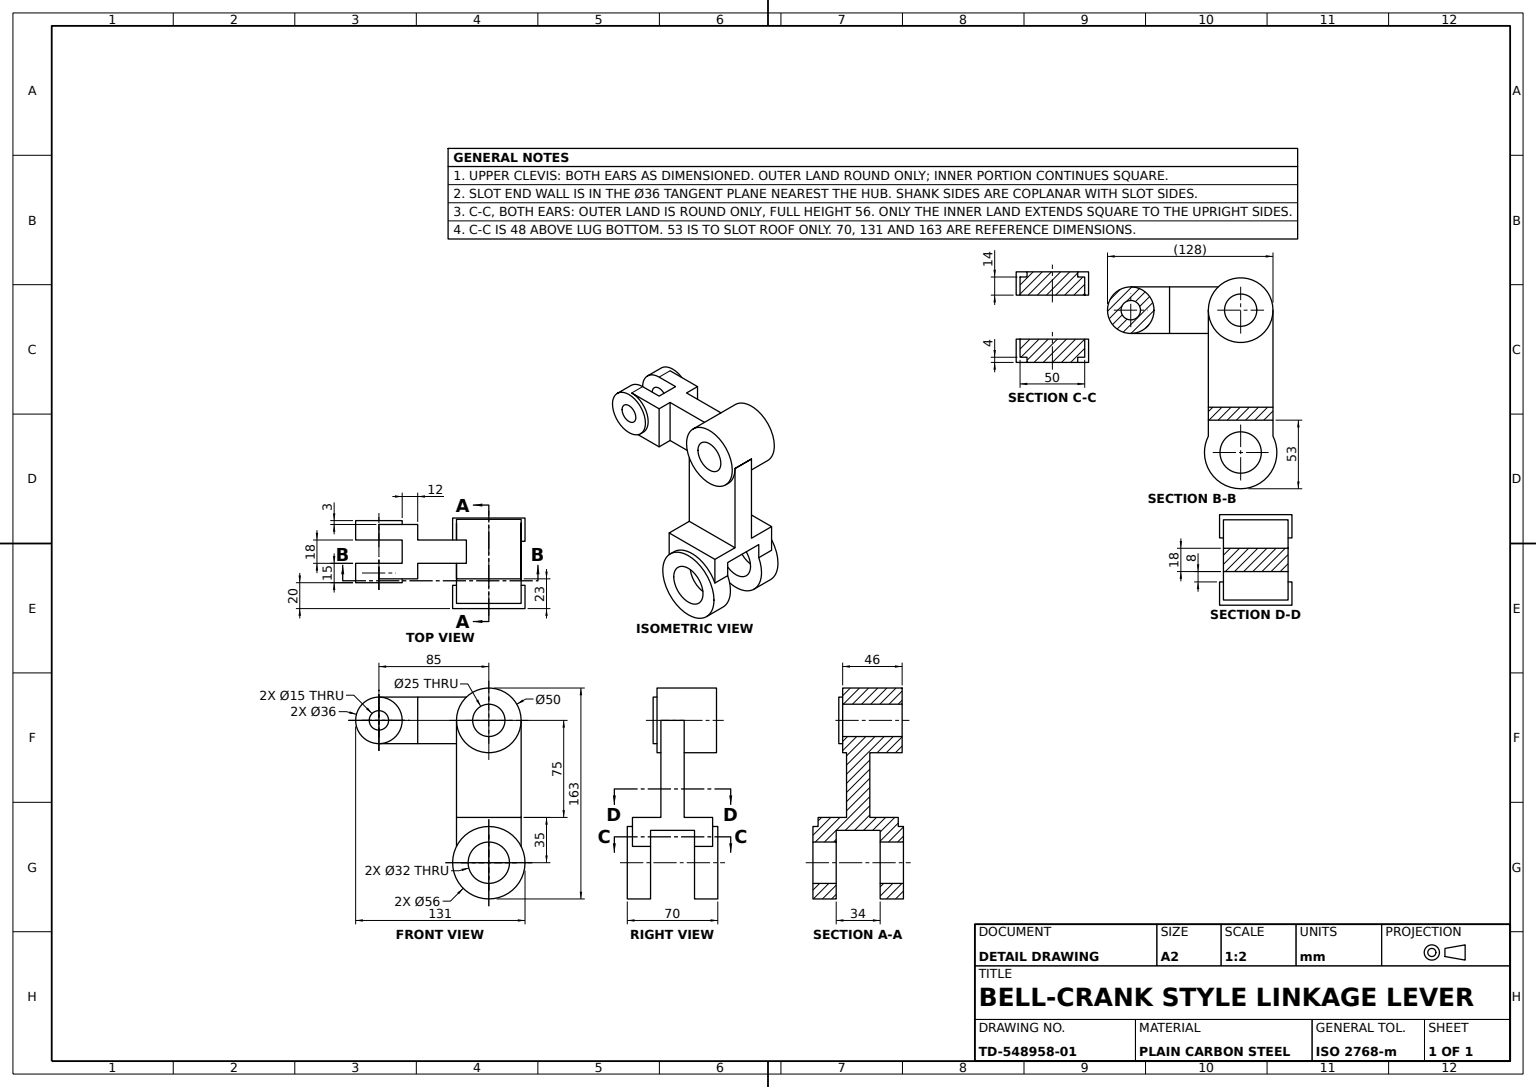
SolidWorks part; units mm, degrees
material "Plain Carbon Steel"
ref_plane "Front Plane" through (0, 0, 0) normal (0, 0, 1) x (1, 0, 0)
ref_plane "Top Plane" through (0, 0, 0) normal (0, 1, 0) x (1, 0, 0)
ref_plane "Right Plane" through (0, 0, 0) normal (1, 0, 0) x (0, 0, -1)
sketch "Front Pivot Eye Sketch" plane through (0, 0, 0) normal (0, 0, 1) x (1, 0, 0)
  circle A0 centre (0, 0) radius 28
  circle A1 centre (0, 0) radius 16
  dimension "D1" = 56
  dimension "D2" = 32
extrude "Front Pivot Eye Ø56xØ32" add sketch "Front Pivot Eye Sketch" against normal blind 18
ref_plane "Plane1" through (0, 0, -52) normal (0, 0, 1) x (1, 0, 0)
sketch "Rear Pivot Eye Sketch" plane through (0, 0, -52) normal (0, 0, 1) x (1, 0, 0)
  circle A0 centre (0, 0) radius 28
  circle A1 centre (0, 0) radius 16
  dimension "D1" = 56
  dimension "D2" = 32
extrude "Rear Pivot Eye Ø56xØ32" add sketch "Rear Pivot Eye Sketch" against normal blind 18 separate body
ref_plane "Plane2" through (0, 35, 0) normal (0, 1, 0) x (1, 0, 0)
sketch "Lower Clevis Block Sketch" plane through (0, 35, 0) normal (0, 1, 0) x (1, 0, 0)
  line L0 (-28, 52) -> (-28, 66)
  line L1 (-28, 70) -> (-28, 52) construction
  line L2 (-28, 66) -> (28, 66)
  line L3 (28, 52) -> (28, 70) construction
  line L4 (28, 66) -> (28, 18)
  line L5 (28, 18) -> (28, 4)
  line L6 (28, 4) -> (-28, 4)
  line L7 (-28, 18) -> (-28, 0) construction
  line L8 (-28, 4) -> (-28, 52)
  dimension "D1" = 48
  dimension "D2" = 48
extrude "Lower Clevis Block 48x48" add sketch "Lower Clevis Block Sketch" against normal blind 18
sketch "Clevis Block Relief Sketch" plane through (0, 0, -4) normal (0, 0, 1) x (1, 0, 0)
  line L0 (-28, 17) -> (-25, 17)
  line L1 (28, 17) -> (25.1243, 17)
  line L2 (-25, 17) -> (-25, 35)
  line L3 (-28, 35) -> (-28, 17)
  line L4 (-28, 17) -> (-28, 35) construction
  line L5 (-28, 17) -> (-22.2486, 17) construction
  line L6 (-28, 35) -> (28, 35) construction
  line L7 (-25, 35) -> (-28, 35)
  line L8 (28, 35) -> (28, 17)
  line L10 (22.2486, 17) -> (28, 17) construction
  line L11 (25.1243, 17) -> (25.0043, 17)
  line L12 (25.0043, 17) -> (25.0043, 35)
  line L13 (25.0043, 35) -> (28, 35)
  dimension "D1" = 3
  dimension "D2" = 2.9957
  dimension "D3" = 2.9957
extrude "Clevis Block Relief Cut" cut sketch "Clevis Block Relief Sketch" against normal through all
sketch "Lower Clevis Slot Sketch" plane through (-25, 0, 0) normal (-1, 0, 0) x (0, 0, 1)
  line L1 (-52, 17) -> (-18, 17)
  line L2 (-52, 17) -> (-52, 25)
  line L3 (-52, 25) -> (-18, 25)
  line L4 (-18, 17) -> (-18, 25)
  dimension "D1" = 34
  dimension "D2" = 8
extrude "Lower Clevis Slot 34x8" cut sketch "Lower Clevis Slot Sketch" against normal through all
sketch "Lower Web Plate Sketch" plane through (0, 17, 0) normal (0, -1, 0) x (1, 0, 0)
  line L0 (22.2486, -4) -> (22.2486, -18) construction
  line L1 (-25, -66) -> (-22.2486, -66)
  line L2 (-25, -66) -> (-25, -52)
  line L3 (-25, -52) -> (-22.2486, -52)
  line L4 (-22.2486, -66) -> (-22.2486, -52)
  line L5 (-25, -18) -> (-22.2486, -18)
  line L6 (-25, -18) -> (-25, -4)
  line L7 (-25, -4) -> (-22.2486, -4)
  line L8 (-22.2486, -18) -> (-22.2486, -4)
  line L9 (22.2486, -4) -> (25.0043, -4)
  line L10 (22.2486, -4) -> (22.2486, -18)
  line L11 (22.2486, -18) -> (25.0043, -18)
  line L12 (25.0043, -4) -> (25.0043, -18)
  line L13 (22.2486, -4) -> (25.0043, -4) construction
  line L15 (22.2486, -52) -> (25.0043, -52)
  line L16 (22.2486, -52) -> (22.2486, -66)
  line L17 (22.2486, -66) -> (25.0043, -66)
  line L18 (25.0043, -52) -> (25.0043, -66)
extrude "Lower Web Plate 5mm" add sketch "Lower Web Plate Sketch" along normal blind 5
sketch "Main Arm Sketch" plane through (0, 35, 0) normal (0, 1, 0) x (1, 0, 0)
  line L0 (-25, 66) -> (-25, 4) construction
  line L1 (-25, 44) -> (25.0043, 44)
  line L2 (-25, 44) -> (-25, 26)
  line L3 (-25, 26) -> (25.0043, 26)
  line L4 (25.0043, 44) -> (25.0043, 26)
  line L5 (25.0043, 4) -> (25.0043, 66) construction
  point P8 (-25, 35)
  dimension "D1" = 9
  dimension "D2" = 18
extrude "Main Arm 9x18" add sketch "Main Arm Sketch" along normal blind 75
ref_plane "Plane4" through (0, 0, -23) normal (0, 0, 1) x (1, 0, 0)
sketch "Upper Pivot Hub Sketch" plane through (0, 0, -23) normal (0, 0, 1) x (1, 0, 0)
  line L0 (-25, 110) -> (25.0043, 110) construction
  circle A0 centre (0.0021, 110) radius 25
  circle A1 centre (0.0021, 110) radius 12.5
  dimension "D1" = 50
  dimension "D2" = 25
extrude "Upper Pivot Hub Ø50xØ25" add sketch "Upper Pivot Hub Sketch" against normal blind 46
sketch "Hub Bore Sketch" plane through (0, 0, -26) normal (0, 0, 1) x (1, 0, 0)
  line L0 (-12.4979, 110) -> (12.5021, 110) construction
  circle A0 centre (0.0021, 110) radius 12.5
  dimension "D1" = 25
extrude "Hub Bore Through Cut Ø25" cut sketch "Hub Bore Sketch" against normal through all
ref_plane "Plane5" through (0, 0, -20) normal (0, 0, 1) x (1, 0, 0)
sketch "Upper Arm Sketch" plane through (0, 0, -20) normal (0, 0, 1) x (1, 0, 0)
  line L0 (0.0021, 122.5) -> (0.0021, 110) construction
  circle A0 centre (-84.9979, 110) radius 18
  circle A1 centre (-84.9979, 110) radius 7.5
  circle A2 centre (0.0021, 110) radius 12.5 construction
  dimension "D1" = 36
  dimension "D2" = 15
  dimension "D3" = 0
  dimension "D4" = 85
extrude "Upper Arm 36x15" add sketch "Upper Arm Sketch" against normal blind 15 separate body
ref_plane "Plane6" through (0, 0, -53) normal (0, 0, 1) x (1, 0, 0)
sketch "Upper Arm Extension Sketch" plane through (0, 0, -53) normal (0, 0, 1) x (1, 0, 0)
  circle A0 centre (-84.9979, 110) radius 18
  circle A1 centre (-84.9979, 110) radius 7.5
  dimension "D1" = 36
  dimension "D2" = 15
extrude "Upper Arm Extension 36x15" add sketch "Upper Arm Extension Sketch" against normal blind 15 separate body
ref_plane "Plane7" through (0, 128, 0) normal (0, 1, 0) x (1, 0, 0)
sketch "Upper Clevis Head Sketch" plane through (0, 128, 0) normal (0, 1, 0) x (1, 0, 0)
  line L0 (-84.9979, 53) -> (-84.9979, 65)
  line L1 (-102.9979, 53) -> (-66.9979, 53) construction
  line L2 (-84.9979, 65) -> (-54.9979, 65)
  line L3 (-54.9979, 65) -> (-54.9979, 53)
  line L4 (-54.9979, 53) -> (-4.7457, 53)
  line L5 (-4.7457, 53) -> (-4.7457, 35)
  line L6 (-4.7457, 35) -> (-54.9979, 35)
  line L7 (-54.9979, 35) -> (-54.9979, 23)
  line L8 (-54.9979, 23) -> (-84.9979, 23)
  line L9 (-84.9979, 23) -> (-84.9979, 35)
  line L10 (-77.4979, 35) -> (-92.4979, 35) construction
  line L11 (-84.9979, 35) -> (-66.9979, 35)
  line L12 (-66.9979, 35) -> (-102.9979, 35) construction
  line L13 (-66.9979, 35) -> (-66.9979, 53)
  line L14 (-66.9979, 53) -> (-84.9979, 53)
  dimension "D1" = 18
  dimension "D2" = 50.2521
  dimension "D3" = 12
  dimension "D4" = 30
  dimension "D5" = 12
  dimension "D6" = 12
extrude "Upper Clevis Head" add sketch "Upper Clevis Head Sketch" against normal blind 36
sketch "Upper Clevis Slot Sketch" plane through (0, 0, -23) normal (0, 0, 1) x (1, 0, 0)
  line L0 (-84.9979, 102.5) -> (-84.9979, 117.5) construction
  circle A0 centre (0.0021, 110) radius 12.5
  circle A1 centre (-84.9979, 110) radius 7.5
  dimension "D1" = 25
extrude "Upper Clevis Slot 25" cut sketch "Upper Clevis Slot Sketch" against normal through all
